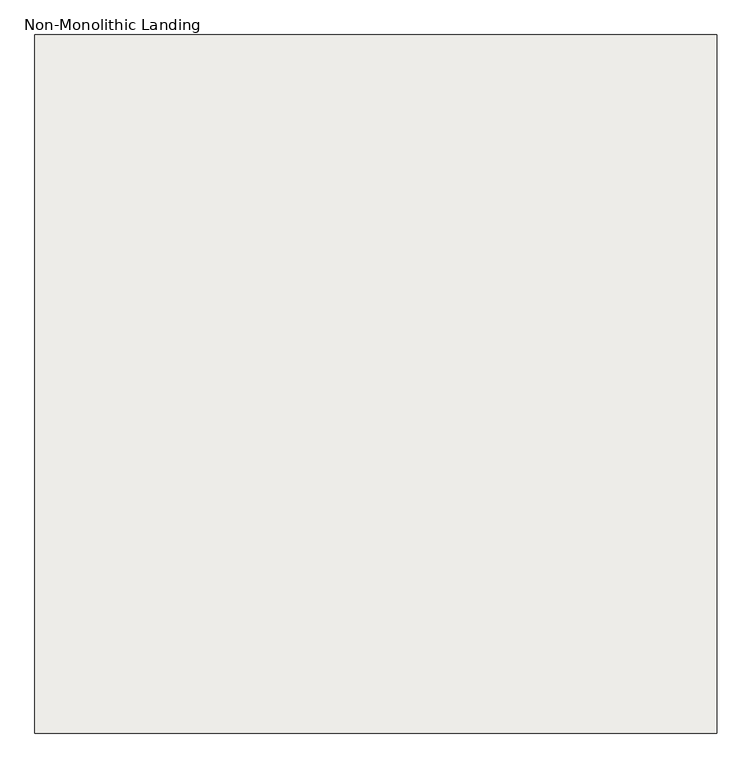
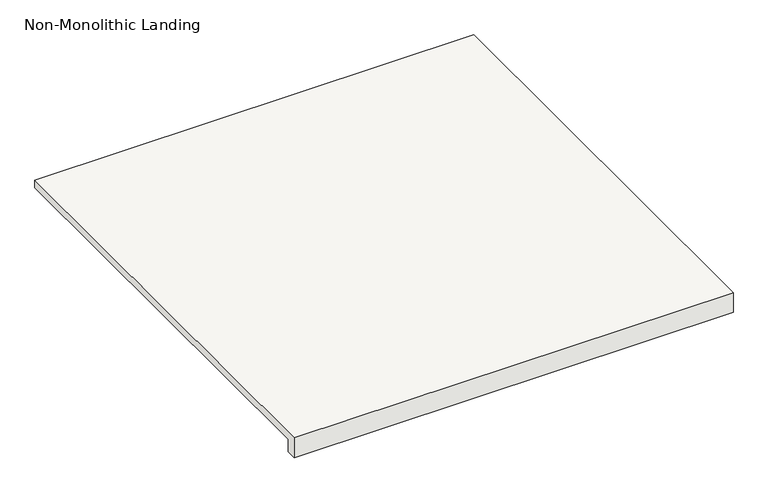
"""IFC4 building model written with IfcOpenShell, lengths in millimetres: slab geometry, Non-Monolithic Landing."""

from ifc_helpers import new_model, si_unit, origin, place, context, project, spatial, faceted_brep, source, transform, mapped, element, save


def non_monolithic_landing_caa31a54(model_context):
    return source(origin(), model_context, "Body", "Brep", [
        faceted_brep([(17678.7916032, 6221.9241878, 857.25), (17704.1916032, 6221.9241878, 831.85), (17704.1916032, 5155.1241878, 831.85), (17678.7916032, 5155.1241878, 857.25), (17678.7916032, 5129.7241878, 876.3), (18745.5916032, 5129.7241878, 876.3), (18745.5916032, 5155.1241878, 876.3), (18745.5916032, 6221.9241878, 876.3), (17678.7916032, 6221.9241878, 876.3), (17704.1916032, 5155.1241878, 825.5), (17704.1916032, 6221.9241878, 825.5), (18745.5916032, 6221.9241878, 825.5), (18745.5916032, 5155.1241878, 825.5), (18745.5916032, 5129.7241878, 825.5), (17678.7916032, 5129.7241878, 825.5), (17678.7916032, 5155.1241878, 825.5)], [[[0, 1, 2, 3]], [[4, 5, 6, 7, 8]], [[9, 10, 11, 12, 13, 14, 15]], [[10, 9, 2, 1]], [[9, 15, 3, 2]], [[4, 8, 0, 3, 15, 14]], [[5, 4, 14, 13]], [[6, 5, 13, 12]], [[7, 6, 12, 11]], [[8, 7, 11, 10, 1, 0]]]),
    ])


if __name__ == "__main__":
    model = new_model("IFC4")
    model_context = context("Model", 3, world=origin())
    ifc_project = project(units=[si_unit("LENGTHUNIT", "METRE", prefix="MILLI")], contexts=[model_context])
    site = spatial("IfcSite", under=ifc_project)
    building = spatial("IfcBuilding", under=site)
    placement = place(None, origin())
    non_monolithic_landing_shape = non_monolithic_landing_caa31a54(model_context)
    element("IfcSlab", 1, ObjectType="Non-Monolithic Landing", at=placement, inside=building, context=model_context, shape_type="MappedRepresentation", body=[
        mapped(non_monolithic_landing_shape, transform((0.0, 0.0, 0.0), x_axis=(1.0, 0.0, 0.0), y_axis=(0.0, 1.0, 0.0), z_axis=(0.0, 0.0, 1.0))),
    ])
    save(model, "model.ifc")
